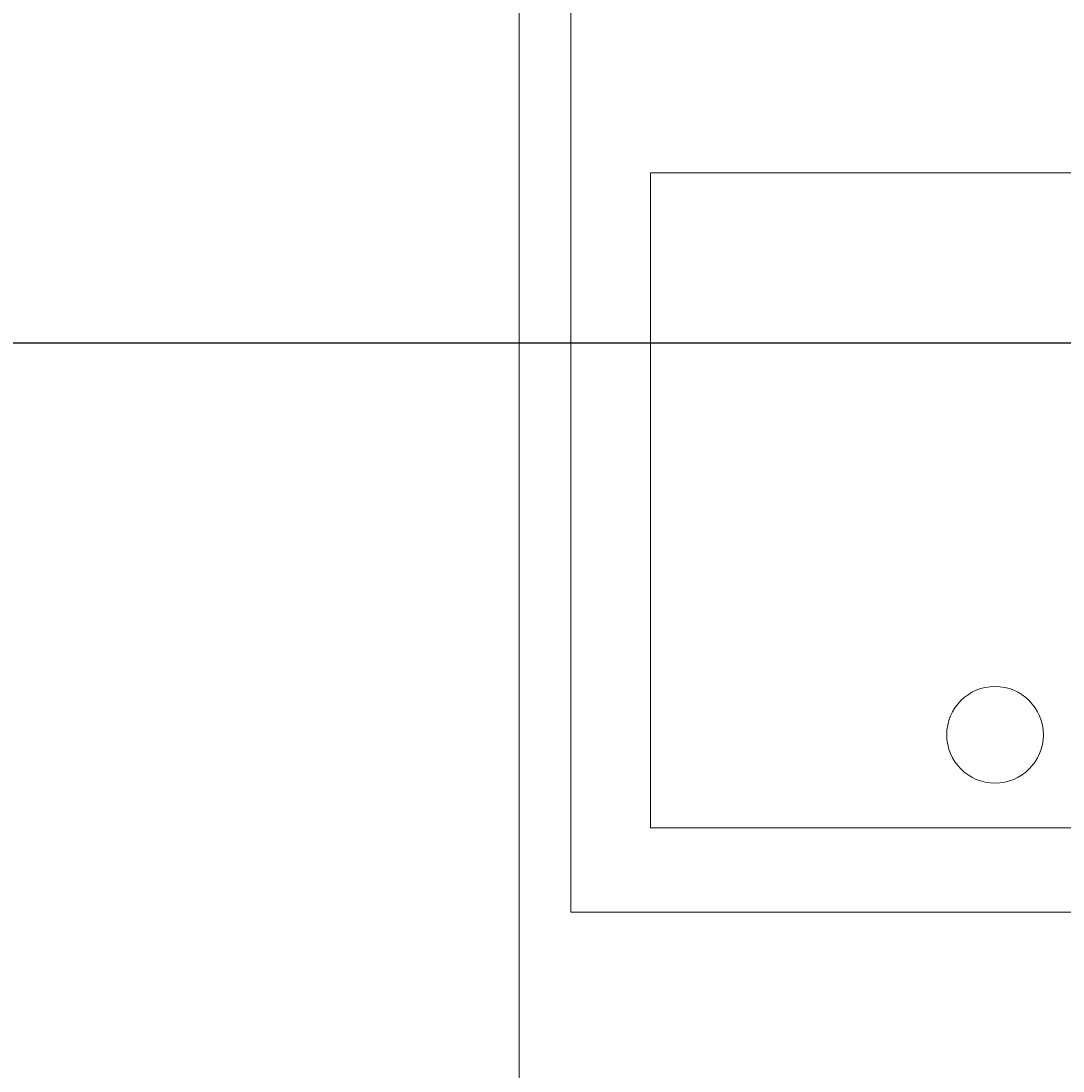
# Model space of a CAD drawing. Units: inches. Extents: x 1568 to 2529, y 2149 to 2897.
# Tile 10 of 16: x 1929 to 1953, y 2434 to 2459. Entities that reach past the tile are written whole.
import ezdxf

# ---------------------------------------------------------------- set-up
doc = ezdxf.new("R2010")
doc.units = ezdxf.units.IN
doc.layers.add('A-ANNO-DIMS', color=2, linetype='Continuous', lineweight=18)
doc.layers.add('A-FLOR-FIXT', color=9, linetype='Continuous', lineweight=18)
doc.styles.get("Standard").update_dxf_attribs({"font": 'arial.ttf'})
doc.dimstyles.get("Standard").update_dxf_attribs({"dimtxt": 0.18, "dimasz": 0.18, "dimexe": 0.18, "dimexo": 0.0625, "dimgap": 0.09, "dimtad": 0, "dimtih": 1, "dimtoh": 1, "dimdec": 4, "dimzin": 0, "dimdsep": 46, "dimtxsty": 'Standard', "dimcen": 0.09, "dimadec": 0, "dimazin": 0, "dimtfac": 1, "dimtdec": 4, "dimtofl": 0, "dimtmove": 0, "dimatfit": 3, "dimfxl": 1, "dimtolj": 1, "dimtzin": 0, "dimarcsym": 0})

# ---------------------------------------------------------------- blocks, each defined once
blk = doc.blocks.new('*D32')
at = {"layer": 'A-ANNO-DIMS', "color": 0, "lineweight": -2, "transparency": 16777216}
for p, q in [((1964.551, 2792.469), (1964.551, 2165.502)), ((1904.551, 2753.401), (1904.551, 2165.502)), ((1904.731, 2165.682), (1934.332, 2165.682)), ((1964.371, 2165.682), (1934.77, 2165.682))]:
    blk.add_line(p, q, dxfattribs=at)
at = {"layer": 'A-ANNO-DIMS', "color": 0, "transparency": 16777216}
for points in [[(1904.731, 2165.712), (1904.731, 2165.652), (1904.551, 2165.682)], [(1964.371, 2165.712), (1964.371, 2165.652), (1964.551, 2165.682)]]:
    blk.add_solid(points, dxfattribs=at)
at = {"layer": 'Defpoints', "color": 0, "transparency": 16777216}
for p in [(1964.551, 2792.532), (1904.551, 2753.463), (1964.551, 2165.682)]:
    blk.add_point(p, dxfattribs=at)
at = {"layer": 'A-ANNO-DIMS', "color": 0, "transparency": 16777216, "insert": (1934.551, 2165.682), "char_height": 0.18, "attachment_point": 5}
blk.add_mtext('\\A1;60', dxfattribs=at)
blk = doc.blocks.new('*D35')
at = {"layer": 'A-ANNO-DIMS', "color": 0, "lineweight": -2, "transparency": 16777216}
for p, q in [((1759.113, 2451.227), (2009.61, 2451.227)), ((2009.43, 2451.047), (2009.43, 2431.409)), ((2009.43, 2411.407), (2009.43, 2431.045)), ((1759.113, 2411.227), (2009.61, 2411.227))]:
    blk.add_line(p, q, dxfattribs=at)
at = {"layer": 'A-ANNO-DIMS', "color": 0, "transparency": 16777216}
for points in [[(2009.4, 2451.047), (2009.46, 2451.047), (2009.43, 2451.227)], [(2009.4, 2411.407), (2009.46, 2411.407), (2009.43, 2411.227)]]:
    blk.add_solid(points, dxfattribs=at)
at = {"layer": 'Defpoints', "color": 0, "transparency": 16777216}
for p in [(1759.051, 2451.227), (2009.43, 2451.227), (1759.051, 2411.227)]:
    blk.add_point(p, dxfattribs=at)
at = {"layer": 'A-ANNO-DIMS', "color": 0, "transparency": 16777216, "insert": (2009.43, 2431.227), "char_height": 0.18, "attachment_point": 5}
blk.add_mtext('\\A1;40', dxfattribs=at)

msp = doc.modelspace()

# ---------------------------------------------------------------- linework, layer by layer
at = {"layer": 'A-FLOR-FIXT'}
msp.add_line((1940.5509, 2471.532), (1940.5509, 2339.532), dxfattribs=at)
for points in [[(1941.7397, 2469.6671), (1961.4644, 2469.6671), (1961.4644, 2438.1142), (1941.7397, 2438.1142)], [(1943.5781, 2440.0573), (1959.4492, 2440.0573), (1959.4492, 2455.1398), (1943.5781, 2455.1398)]]:
    msp.add_lwpolyline(points, close=True, dxfattribs=at)
msp.add_circle((1951.5106, 2442.2007), 1.1131, dxfattribs=at)

# ---------------------------------------------------------------- dimensions: what is measured, and where the dimension line sits
at = {"layer": 'A-ANNO-DIMS'}
dim = msp.add_linear_dim(base=(1964.5509, 2165.682), p1=(1904.5509, 2753.4635), p2=(1964.5509, 2792.532), dimstyle='Standard', override={"dimdec": 0, "dimlfac": 1, "dimrnd": 0, "dimzin": 0, "dimdsep": 46, "dimlunit": 2}, dxfattribs=at)
dim.commit()
dim.dimension.update_dxf_attribs({"geometry": '*D32', "text_midpoint": (1934.5509, 2165.682)})
dim = msp.add_linear_dim(base=(2009.4302, 2451.2271), p1=(1759.0509, 2411.2271), p2=(1759.0509, 2451.2271), angle=90, dimstyle='Standard', override={"dimdec": 0, "dimlfac": 1, "dimrnd": 0, "dimzin": 0, "dimdsep": 46, "dimlunit": 2}, dxfattribs=at)
dim.commit()
dim.dimension.update_dxf_attribs({"geometry": '*D35', "text_midpoint": (2009.4302, 2431.2271)})

doc.saveas('drawing.dxf')
